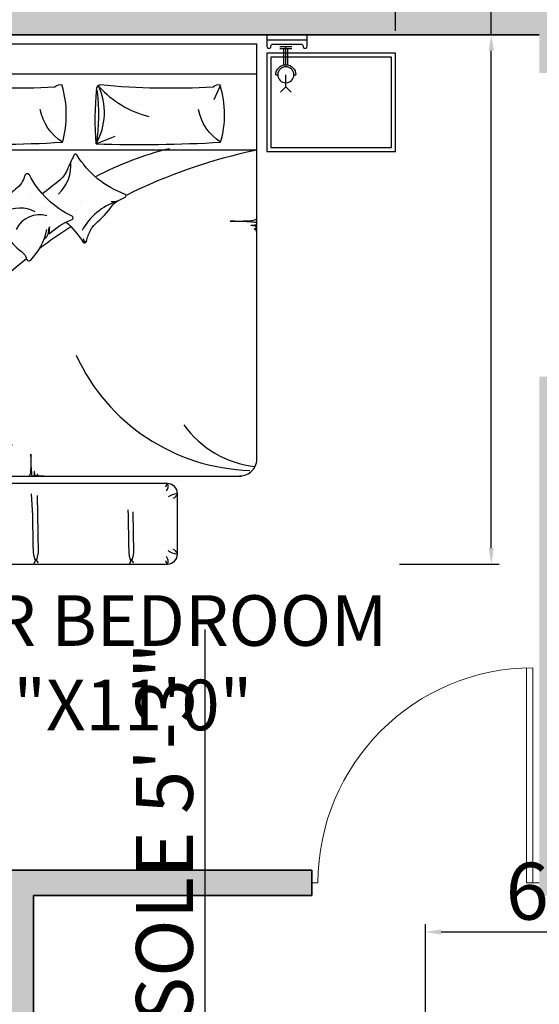
# Model space of a CAD drawing. Units: inches. Extents: x 3592 to 4861, y 1650 to 2243.
# Tile 23 of 30: x 4109 to 4191, y 2003 to 2159. Entities that reach past the tile are written whole.
import ezdxf

# ---------------------------------------------------------------- set-up
doc = ezdxf.new("R2010")
doc.units = ezdxf.units.IN
for name, color, linetype, lineweight in [('A-ANNO-DIMS', 2, 'Continuous', 13), ('A-AREA-IDEN', 7, 'Continuous', 18), ('A-DOOR', 3, 'Continuous', 20), ('A-FURN', 9, 'Continuous', 13), ('A-WALL', 7, 'Continuous', 35)]:
    doc.layers.add(name, color=color, linetype=linetype, lineweight=lineweight)
doc.layers.add('A-WALL-PATT', color=252, linetype='Continuous', lineweight=13, true_color=0x939598)
for name, color, linetype in [('CEIL', 4, 'Continuous'), ('ELEC', 4, 'Continuous'), ('FUR', 42, 'Continuous'), ('wood', 26, 'Continuous')]:
    doc.layers.add(name, color=color, linetype=linetype)
doc.styles.get("Standard").update_dxf_attribs({"font": 'arial.ttf'})
doc.dimstyles.new('ISO-25', dxfattribs={"dimtxt": 9, "dimasz": 2.5, "dimexe": 1.25, "dimexo": 0.625, "dimtad": 1, "dimlunit": 3, "dimtxsty": 'Standard', "dimcen": 2.5, "dimadec": 0, "dimazin": 0, "dimtfac": 1, "dimtmove": 0, "dimatfit": 3, "dimfxl": 1, "dimarcsym": 0})

# ---------------------------------------------------------------- blocks, each defined once
blk = doc.blocks.new('1')
for p, q in [((3628.27, 1890.86), (3628.27, 1924.86)), ((3629.27, 1890.86), (3629.27, 1924.86)), ((3627.27, 1890.86), (3629.27, 1890.86)), ((3662.27, 1890.86), (3663.27, 1890.86))]:
    blk.add_line(p, q)
blk.add_arc((3628.27, 1890.86), 34, 0, 90)
blk = doc.blocks.new('*X20')
at = {"color": 0}
for p, q in [((3155.9, 8182.9), (3155.9, 8182.9)), ((3147.8, 8143.4), (3147.8, 8143.4)), ((3283, 8049.6), (3283, 8049.6)), ((3209.5, 8023.9), (3209.5, 8023.9)), ((3251.6, 7997), (3251.6, 7997)), ((3154.1, 7950.7), (3154.1, 7950.7))]:
    blk.add_line(p, q, dxfattribs=at)
blk = doc.blocks.new('*X19')
at = {"color": 0}
for p, q in [((3155.9, 8182.9), (3155.9, 8182.9)), ((3139.8, 7939.7), (3139.8, 7939.7))]:
    blk.add_line(p, q, dxfattribs=at)
blk = doc.blocks.new('*X18')
at = {"color": 0}
for p, q in [((3155.9, 8182.9), (3155.9, 8182.9)), ((3139.8, 7939.7), (3139.8, 7939.7))]:
    blk.add_line(p, q, dxfattribs=at)
blk = doc.blocks.new('*X17')
at = {"color": 0}
for p, q in [((3163, 7776.2), (3163, 7776.2)), ((3422.2, 7761.3), (3422.2, 7761.3)), ((3244.3, 7698.6), (3244.3, 7698.6)), ((3340.3, 7689.4), (3340.3, 7689.4)), ((3236.2, 7675.7), (3236.2, 7675.7))]:
    blk.add_line(p, q, dxfattribs=at)
blk = doc.blocks.new('BED1')
for p, q in [((0, -1000), (0, 800)), ((150, 800), (0, 800)), ((150, 800), (150, -1000)), ((2058.7, 800), (150, 800)), ((528, 800), (528, -1000)), ((211.8, 614.9), (277.5, 585.4)), ((2537.2, 404.9), (2237.2, 404.9)), ((2187.2, 354.9), (2187.2, -545.1)), ((2587.2, -545.1), (2587.2, 354.9)), ((2566.3, 178.5), (2565.2, 177.4)), ((2582, 188.1), (2565.4, 174.8)), ((2565.4, 174.8), (2585.7, 165.4)), ((2582, -287.1), (2565.4, -300.5)), ((2566.3, -296.8), (2565.2, -297.9)), ((2565.4, -300.5), (2585.7, -309.9)), ((2237.2, -595.1), (2537.2, -595.1)), ((150, -1000), (0, -1000)), ((150, -1000), (2063.5, -1000))]:
    blk.add_line(p, q)
for points in [[(934, 797.9), (930.9, 797.7), (928.3, 797.4), (926.3, 796.9), (924.9, 796.3), (923.8, 795.6), (923.1, 794.8), (922.7, 793.8), (922.5, 792.7), (922.4, 791.5), (922.5, 790.3), (922.6, 789.2), (922.6, 788.3), (922.6, 787.6), (922.4, 787.3), (922, 787.4), (921.4, 787.9), (920.6, 788.9), (919.5, 790.2), (918.4, 791.6), (917.1, 793.1), (915.9, 794.6), (914.6, 796), (913.3, 797.1), (912.2, 797.9), (911.1, 798.3), (910.1, 798.4), (909.2, 798), (908.3, 797.1), (907.5, 795.8), (906.8, 793.9), (906, 791.4), (905.4, 788.5), (904.8, 785.2), (904.2, 781.7), (903.7, 778.4), (903.2, 775.4), (902.8, 772.9), (902.5, 771.3), (902.3, 770.6), (902.1, 771.2), (902, 772.8), (901.8, 775.2), (901.7, 778.1), (901.5, 781.5), (901.2, 785), (900.8, 788.4), (900.2, 791.5), (899.5, 794.1), (898.6, 796.2), (897.6, 797.9), (896.5, 799.2), (895.3, 800), (894.1, 800.5), (893, 800.7), (891.9, 800.5), (890.9, 800.1), (890, 799), (889.1, 797.1), (888.3, 794), (887.6, 789.3), (886.9, 782.9), (886.2, 774.2), (885.5, 763.1), (884.8, 749.5), (884.2, 734.2), (883.6, 718.3), (883, 702.8), (882.5, 688.8), (882, 677.5), (881.7, 669.8), (881.5, 666.9), (881.3, 669.4), (881.3, 676.7), (881.3, 687.8), (881.2, 701.5), (881.1, 716.8), (880.8, 732.6), (880.2, 748), (879.4, 761.8), (878.3, 773.2), (876.9, 782.2), (875.1, 789.2), (872.9, 794.4), (870.3, 798), (869, 799)], [(2150, -913.5), (2150, 723.2)], [(2327.6, 182.3), (2530, 185.9), (2550.8, 181.9), (2561.7, 179), (2566, 176.7), (2566.9, 174.4), (2566.3, 171.9), (2562, 169.2), (2550.3, 166.5), (2527.7, 163.9), (2490.6, 161.8), (2345.5, 160.2), (2317.8, 158.5)], [(494.7, 3.1), (458.9, 95.3)], [(2149.7, -259.9), (2150, -268.4), (2150.1, -274.1), (2150.1, -278.1), (2150, -281.4), (2149.8, -284), (2149.5, -286.1), (2149.1, -287.8), (2148.7, -289), (2148.1, -289.9), (2147.4, -290.5), (2146.6, -290.8), (2145.6, -291), (2144.6, -291), (2143.6, -291), (2142.7, -290.9), (2141.9, -290.9), (2141.4, -290.9), (2141.1, -291), (2141.2, -291.4), (2141.7, -291.9), (2142.5, -292.6), (2143.5, -293.4), (2144.7, -294.4), (2146, -295.4), (2147.2, -296.5), (2148.4, -297.6), (2149.3, -298.6), (2150, -299.6), (2150.3, -300.5), (2150.4, -301.3), (2150, -302.1), (2149.3, -302.8), (2148.2, -303.5), (2146.6, -304.1), (2144.6, -304.7), (2142.1, -305.2), (2139.3, -305.7), (2136.5, -306.2), (2133.7, -306.6), (2131.2, -307), (2129.2, -307.3), (2127.8, -307.6), (2127.3, -307.8), (2127.7, -308), (2129, -308.1), (2131, -308.2), (2133.5, -308.3), (2136.3, -308.5), (2139.2, -308.7), (2142, -309), (2144.6, -309.5), (2146.8, -310.1), (2148.6, -310.9), (2150, -311.7), (2151, -312.7), (2151.7, -313.6), (2152.1, -314.6), (2152.3, -315.6), (2152.2, -316.5), (2151.8, -317.3), (2150.9, -318.1), (2149.3, -318.8), (2146.7, -319.4), (2142.8, -320), (2137.4, -320.6), (2130.2, -321.2), (2121, -321.8), (2109.7, -322.3), (2096.9, -322.9), (2083.6, -323.4), (2070.7, -323.9), (2059.1, -324.3), (2049.6, -324.7), (2043.2, -325), (2040.8, -325.2), (2042.9, -325.3), (2049, -325.3), (2058.2, -325.3), (2069.6, -325.4), (2082.3, -325.5), (2095.6, -325.8), (2108.4, -326.2), (2119.9, -326.8), (2129.4, -327.8), (2136.9, -329), (2142.7, -330.5), (2147, -332.3), (2150, -334.4), (2150.9, -335.6)], [(2246.5, -294.4), (2530, -289.4), (2550.8, -293.4), (2561.7, -296.3), (2566, -298.6), (2566.9, -300.8), (2566.3, -303.4), (2562, -306.1), (2550.3, -308.8), (2527.7, -311.3), (2490.6, -313.5), (2345.5, -315), (2238.6, -321.8)], [(1733.7, -998.3), (1731.1, -998.1), (1729, -997.8), (1727.4, -997.4), (1726.1, -997), (1725.2, -996.4), (1724.7, -995.7), (1724.3, -994.8), (1724.1, -993.9), (1724.1, -992.9), (1724.1, -991.9), (1724.2, -991), (1724.2, -990.2), (1724.2, -989.7), (1724.1, -989.4), (1723.8, -989.5), (1723.2, -990), (1722.5, -990.8), (1721.7, -991.8), (1720.7, -993), (1719.7, -994.3), (1718.6, -995.5), (1717.5, -996.6), (1716.5, -997.6), (1715.5, -998.3), (1714.6, -998.6), (1713.8, -998.6), (1713, -998.3), (1712.3, -997.6), (1711.7, -996.5), (1711, -994.9), (1710.4, -992.9), (1709.9, -990.4), (1709.4, -987.6), (1708.9, -984.8), (1708.5, -982), (1708.1, -979.5), (1707.8, -977.4), (1707.5, -976.1), (1707.3, -975.5), (1707.1, -976), (1707, -977.3), (1706.9, -979.3), (1706.8, -981.8), (1706.7, -984.6), (1706.4, -987.5), (1706.1, -990.3), (1705.6, -992.9), (1705, -995.1), (1704.2, -996.9), (1703.4, -998.3), (1702.4, -999.3), (1701.5, -1000), (1700.5, -1000.4), (1699.6, -1000.6), (1698.7, -1000.4), (1697.8, -1000.1), (1697, -999.2), (1696.3, -997.6), (1695.7, -995), (1695.1, -991.1), (1694.5, -985.7), (1693.9, -978.5), (1693.3, -969.3), (1692.8, -957.9), (1692.2, -945.2), (1691.7, -931.9), (1691.2, -919), (1690.8, -907.4), (1690.4, -897.9), (1690.1, -891.5), (1689.9, -889.1), (1689.8, -891.2), (1689.8, -897.3), (1689.8, -906.5), (1689.7, -917.9), (1689.6, -930.6), (1689.4, -943.8), (1688.9, -956.6), (1688.3, -968.1), (1687.3, -977.6), (1686.1, -985.2), (1684.6, -991), (1682.8, -995.3), (1680.7, -998.3), (1679.6, -999.2)]]:
    blk.add_lwpolyline(points)
for points in [[(489.2, 619.6, 0.144019), (207.6, 617.9, 0.248643)], [(205.5, 619.6, 0.267769), (215.1, 582.4, -0.037739), (204.3, 21.8, 0.684696), (236.7, 5.5, -0.060702), (497.2, 0.1, -0.046649), (225.9, 3.1, -1.318436)], [(497.2, 0.1, 0.021276), (489.2, 619.6, -0.206383), (326.6, 509.4, 0.237198)], [(211.8, 12.8, 0.143972), (361.6, 262.9, 1.292232)], [(886.4, -150, -0.069098), (985, -66.5, 0.658965), (982.1, -48.7, -0.049789), (927.4, -29, -0.103757), (896.6, -5.4, 0.055725), (800.9, 83.3, -0.11866), (782.7, 104.9, 0.016811), (761.6, 143.9, 0.70791), (748.3, 144, -0.16964), (551.9, -96.6, 0.664036), (554, -110.7, 0.023706), (627, -144.7, -0.134834), (683.2, -188, 0.012748), (746.3, -267.4)], [(969.1, -259.1, 0.263265), (936.3, -236.9, -0.026108), (909.2, -233.2, 0.027613), (945.1, -234.2, -0.089259), (872.7, -120, 0.662242), (857.6, -119.3, -0.162037), (651.8, -332.7, 0.676499), (654, -354.5, -0.160513), (722.9, -401.5, 0.07473), (773.5, -450.3, -0.187721), (845.5, -559.9, 0.70791), (858.8, -561.4, -0.010003), (898.6, -497.3, -0.113819), (947.3, -450.2, 0.099539), (1032.5, -372.4, -0.173425), (1070.9, -346.4, 0.589988), (1076.2, -326.1, 0.137312), (923.9, -245.9, 0.137312)], [(205.5, -168.2, 0.267769), (215.1, -205.4, -0.037739), (204.3, -766, 0.684696), (236.7, -782.3, -0.060702), (497.2, -787.7, -0.046649), (225.9, -784.7, -1.318436)], [(489.2, -168.2, 0.144019), (207.6, -169.9, 0.248643)], [(497.2, -787.7, 0.021276), (489.2, -168.2, -0.206383), (326.6, -278.4, 0.237198)], [(1446, -733.4, -0.095039), (652.8, -1001.7)]]:
    blk.add_lwpolyline(points, format="xyb")
for centre, radius, start, end in [((3208.8, 1363.3), 2739.4, 191.8679, 206.3247), ((1608.1, 842.5), 496.3, 305.1901, 354.0206), ((2062.7, 713.7), 86.5, 0, 93.5376), ((1138.6, 793.9), 983.2, 294.6078, 358.3033), ((2237.2, 354.9), 50, 90, 180), ((2321.1, 409.7), 84.5, 185.6196, 217.1396), ((2227.5, 373.5), 32.8, 17.833, 72.8005), ((2546.9, 373.5), 32.8, 107.1995, 162.167), ((2453.3, 409.7), 84.5, 322.8604, 354.3804), ((2537.2, 354.9), 50, 0, 90), ((2098.7, 754.7), 1625, 193.905, 207.8169), ((2201.9, 323.3), 34.8, 50.8413, 114.9586), ((2212.2, 381.5), 36.5, 226.8095, 258.3841), ((2572.5, 323.3), 34.8, 65.0414, 129.1587), ((2562.2, 381.5), 36.5, 281.6159, 313.1905), ((751.8, 88.7), 34.9, 336.8352, 27.7218), ((684.2, 86), 100.3, 353.675, 10.882), ((1074.1, 198.8), 306.1, 197.8602, 241.5122), ((341.4, -277.7), 318.5, 60.7125, 115.009), ((983.7, -79.5), 20.8, 73.7967, 130.4566), ((978.5, -68.6), 14.3, 39.7097, 85.9506), ((602.5, -324), 198.6, 43.2035, 95.0556), ((3208.8, 1363.3), 2739.4, 212.9314, 216.951), ((981.1, -281.8), 131.1, 164.0372, 243.4536), ((980, -379), 163.4, 152.6104, 209.361), ((3208.8, 1363.3), 2739.4, 218.6329, 229.9449), ((2098.7, 754.7), 1625, 226.5887, 246.3156), ((3402.5, -342.9), 1408.5, 182.9917, 205.6819), ((-34.4, -471.2), 376.5, 312.0118, 350.9635), ((2178, -513.5), 33, 286.1827, 338.1386), ((2188.1, -476.2), 73, 269.4513, 322.8027), ((2562.2, -571.8), 36.5, 46.8095, 78.3841), ((2237.2, -545.1), 50, 180, 270), ((2271.1, -580.9), 35.8, 148.9055, 197.5541), ((2546.9, -563.8), 32.8, 197.833, 252.8005), ((2453.3, -600), 84.5, 5.6196, 37.1396), ((2537.2, -545.1), 50, 270, 0), ((2572.5, -513.6), 34.8, 230.8413, 294.9586), ((375.7, -807.4), 128.2, 17.4073, 88.5129), ((341.4, -1065.5), 318.5, 60.7125, 115.009), ((1929.1, -1126), 250.5, 37.8553, 88.4405), ((2063.5, -913.5), 86.5, 270, 0)]:
    blk.add_arc(centre, radius, start, end)
for name in ['*X19', '*X18', '*X20', '*X17']:
    blk.add_blockref(name, (-2425.3, -8101.4))
blk = doc.blocks.new('APLIQ')
at = {"layer": 'ELEC'}
for p, q in [((0, 0.2), (-0.0261, 0.2261)), ((0, 0.2), (0.0261, 0.2261)), ((0, 0.2), (0, 0.14)), ((-0.05, 0.14), (-0.04, 0.14)), ((0.04, 0.14), (0.05, 0.14)), ((-0.01, 0.09), (-0.01, 0.01)), ((0, 0.09), (0, 0)), ((0.01, 0.09), (0.01, 0.01)), ((-0.03, 0.01), (0.03, 0.01)), ((-0.03, 0), (0.03, 0))]:
    blk.add_line(p, q, dxfattribs=at)
blk.add_circle((0, 0.14), 0.04, dxfattribs=at)
blk.add_arc((0, 0.14), 0.05, 180, 0, dxfattribs=at)
blk = doc.blocks.new('A$C68AE1801')
at = {"layer": 'FUR'}
for points in [[(2.5416, 3.18), (2.5416, 2.54), (2.0516, 2.54), (2.0516, 3.18)], [(2.5216, 3.16), (2.5216, 2.56), (2.0716, 2.56), (2.0716, 3.16)], [(2.5416, 0), (2.5416, 0.64), (2.0516, 0.64), (2.0516, 0)], [(2.5216, 0.02), (2.5216, 0.62), (2.0716, 0.62), (2.0716, 0.02)]]:
    blk.add_lwpolyline(points, close=True, dxfattribs=at)
at = {"layer": 'wood'}
for p, q in [((2.6057, 2.74), (2.6057, 2.54)), ((2.6057, 0.44), (2.6057, 0.64))]:
    blk.add_line(p, q, dxfattribs=at)
for points in [[(2.5657, 2.728), (2.5657, 2.732, -0.414214), (2.5737, 2.74), (2.6321, 2.74), (2.6321, 2.54), (2.5737, 2.54, -0.414214), (2.5657, 2.548), (2.5657, 2.552, -0.414214), (2.5737, 2.56), (2.5777, 2.56, 0.414214), (2.5857, 2.568), (2.5857, 2.712, 0.414214), (2.5777, 2.72), (2.5737, 2.72, -0.414214)], [(2.5657, 0.452), (2.5657, 0.448, 0.414214), (2.5737, 0.44), (2.6321, 0.44), (2.6321, 0.64), (2.5737, 0.64, 0.414214), (2.5657, 0.632), (2.5657, 0.628, 0.414214), (2.5737, 0.62), (2.5777, 0.62, -0.414214), (2.5857, 0.612), (2.5857, 0.468, -0.414214), (2.5777, 0.46), (2.5737, 0.46, 0.414214)]]:
    blk.add_lwpolyline(points, format="xyb", close=True, dxfattribs=at)
at = {"layer": 'CEIL', "rotation": 90}
blk.add_blockref('APLIQ', (2.5736, 2.634), dxfattribs=at)
at = {"layer": 'CEIL', "xscale": -1, "rotation": 90}
blk.add_blockref('APLIQ', (2.5736, 0.546), dxfattribs=at)
at = {"layer": 'FUR', "xscale": 0.001, "yscale": 0.001, "zscale": 0.001, "rotation": 180}
blk.add_blockref('BED1', (2.5872, 1.49), dxfattribs=at)
blk = doc.blocks.new('*D150')
at = {"layer": 'A-ANNO-DIMS', "color": 0, "lineweight": -2, "transparency": 16777216}
for p, q in [((4101.85, 2020.28), (4101.85, 2140.68)), ((4100.04, 2020.28), (4103.1, 2020.28)), ((4101.85, 2006.52), (4101.85, 2017.78)), ((4100.04, 2004.02), (4103.1, 2004.02))]:
    blk.add_line(p, q, dxfattribs=at)
at = {"layer": 'A-ANNO-DIMS', "color": 0, "transparency": 16777216}
for points in [[(4101.43, 2017.78), (4102.27, 2017.78), (4101.85, 2020.28)], [(4101.43, 2006.52), (4102.27, 2006.52), (4101.85, 2004.02)]]:
    blk.add_solid(points, dxfattribs=at)
at = {"layer": 'Defpoints', "color": 0, "transparency": 16777216}
for p in [(4099.41, 2020.28), (4101.85, 2020.28), (4099.41, 2004.02)]:
    blk.add_point(p, dxfattribs=at)
at = {"layer": 'A-ANNO-DIMS', "color": 0, "transparency": 16777216, "insert": (4096.57, 2081.73), "char_height": 9, "attachment_point": 5, "rotation": 90}
blk.add_mtext('BASIN 1\'-4 1/2" TYP.', dxfattribs=at)
blk = doc.blocks.new('*D154')
at = {"layer": 'A-ANNO-DIMS', "color": 0, "lineweight": -2, "transparency": 16777216}
for p, q in [((4067.61, 2156.84), (4067.61, 2172.62)), ((4168.62, 2156.84), (4168.62, 2172.62)), ((4067.61, 2171.37), (3930.45, 2171.37)), ((4166.12, 2171.37), (4070.11, 2171.37))]:
    blk.add_line(p, q, dxfattribs=at)
at = {"layer": 'A-ANNO-DIMS', "color": 0, "transparency": 16777216}
for points in [[(4070.11, 2171.79), (4070.11, 2170.95), (4067.61, 2171.37)], [(4166.12, 2171.79), (4166.12, 2170.95), (4168.62, 2171.37)]]:
    blk.add_solid(points, dxfattribs=at)
at = {"layer": 'Defpoints', "color": 0, "transparency": 16777216}
for p in [(4067.61, 2171.37), (4067.61, 2156.22), (4168.62, 2156.22)]:
    blk.add_point(p, dxfattribs=at)
at = {"layer": 'A-ANNO-DIMS', "color": 0, "transparency": 16777216, "insert": (3997.78, 2176.65), "char_height": 9, "attachment_point": 5}
blk.add_mtext('BED GROUP 8\'-5" TYP.', dxfattribs=at)
blk = doc.blocks.new('*D155')
at = {"layer": 'A-ANNO-DIMS', "color": 0, "lineweight": -2, "transparency": 16777216}
for p, q in [((4183.77, 2156.22), (4183.77, 2242.84)), ((4169.25, 2156.22), (4185.02, 2156.22)), ((4183.77, 2075.11), (4183.77, 2153.72)), ((4169.25, 2072.61), (4185.02, 2072.61))]:
    blk.add_line(p, q, dxfattribs=at)
at = {"layer": 'A-ANNO-DIMS', "color": 0, "transparency": 16777216}
for points in [[(4183.36, 2153.72), (4184.19, 2153.72), (4183.77, 2156.22)], [(4183.36, 2075.11), (4184.19, 2075.11), (4183.77, 2072.61)]]:
    blk.add_solid(points, dxfattribs=at)
at = {"layer": 'Defpoints', "color": 0, "transparency": 16777216}
for p in [(4168.62, 2156.22), (4183.77, 2156.22), (4168.62, 2072.61)]:
    blk.add_point(p, dxfattribs=at)
at = {"layer": 'A-ANNO-DIMS', "color": 0, "transparency": 16777216, "insert": (4178.5, 2200.78), "char_height": 9, "attachment_point": 5, "rotation": 90}
blk.add_mtext('6\'-11 1/2" TYP.', dxfattribs=at)
blk = doc.blocks.new('*D165')
at = {"layer": 'A-ANNO-DIMS', "color": 0, "lineweight": -2, "transparency": 16777216}
for p, q in [((4173.35, 1996.55), (4173.35, 2015.72)), ((4247.08, 1996.55), (4247.08, 2015.72)), ((4175.85, 2014.47), (4244.58, 2014.47))]:
    blk.add_line(p, q, dxfattribs=at)
at = {"layer": 'A-ANNO-DIMS', "color": 0, "transparency": 16777216}
for points in [[(4175.85, 2014.88), (4175.85, 2014.05), (4173.35, 2014.47)], [(4244.58, 2014.88), (4244.58, 2014.05), (4247.08, 2014.47)]]:
    blk.add_solid(points, dxfattribs=at)
at = {"layer": 'Defpoints', "color": 0, "transparency": 16777216}
for p in [(4247.08, 2014.47), (4173.35, 1995.93), (4247.08, 1995.93)]:
    blk.add_point(p, dxfattribs=at)
at = {"layer": 'A-ANNO-DIMS', "color": 0, "transparency": 16777216, "insert": (4210.21, 2019.75), "char_height": 9, "attachment_point": 5}
blk.add_mtext('6\'-1 1/2"', dxfattribs=at)
blk = doc.blocks.new('*D168')
at = {"layer": 'A-ANNO-DIMS', "color": 0, "lineweight": -2, "transparency": 16777216}
for p, q in [((4138.54, 1969.72), (4138.54, 2062.26)), ((4129.71, 1969.72), (4139.79, 1969.72)), ((4138.54, 1909.22), (4138.54, 1967.22)), ((4129.71, 1906.72), (4139.79, 1906.72))]:
    blk.add_line(p, q, dxfattribs=at)
at = {"layer": 'A-ANNO-DIMS', "color": 0, "transparency": 16777216}
for points in [[(4138.12, 1967.22), (4138.95, 1967.22), (4138.54, 1969.72)], [(4138.12, 1909.22), (4138.95, 1909.22), (4138.54, 1906.72)]]:
    blk.add_solid(points, dxfattribs=at)
at = {"layer": 'Defpoints', "color": 0, "transparency": 16777216}
for p in [(4129.09, 1969.72), (4138.54, 1969.72), (4129.09, 1906.72)]:
    blk.add_point(p, dxfattribs=at)
at = {"layer": 'A-ANNO-DIMS', "color": 0, "transparency": 16777216, "insert": (4133.25, 2017.24), "char_height": 9, "attachment_point": 5, "rotation": 90}
blk.add_mtext('CONSOLE 5\'-3"', dxfattribs=at)
blk = doc.blocks.new('*D179')
at = {"layer": 'A-ANNO-DIMS', "color": 0, "lineweight": -2, "transparency": 16777216}
for p, q in [((4092.37, 2010.81), (4092.37, 2193.52)), ((4094.87, 2192.27), (4104.87, 2192.27)), ((4107.37, 2020.84), (4107.37, 2193.52)), ((4107.37, 2192.27), (4134.2, 2192.27))]:
    blk.add_line(p, q, dxfattribs=at)
at = {"layer": 'A-ANNO-DIMS', "color": 0, "transparency": 16777216}
for points in [[(4094.87, 2192.69), (4094.87, 2191.85), (4092.37, 2192.27)], [(4104.87, 2192.69), (4104.87, 2191.85), (4107.37, 2192.27)]]:
    blk.add_solid(points, dxfattribs=at)
at = {"layer": 'Defpoints', "color": 0, "transparency": 16777216}
for p in [(4107.37, 2192.27), (4107.37, 2020.22), (4092.37, 2010.18)]:
    blk.add_point(p, dxfattribs=at)
at = {"layer": 'A-ANNO-DIMS', "color": 0, "transparency": 16777216, "insert": (4122.03, 2197.49), "char_height": 9, "attachment_point": 5}
blk.add_mtext('1\'-3"', dxfattribs=at)

msp = doc.modelspace()

# ---------------------------------------------------------------- hatches: boundary and pattern name
at = {"layer": 'A-WALL-PATT'}
h = msp.add_hatch(color=256, dxfattribs=at)
h.dxf.hatch_style = 1
h.paths.add_polyline_path([(4398.37, 2165.219), (4038.37, 2165.219), (4038.37, 1993.219), (4047.37, 1993.219), (4047.37, 2156.219), (4191.37, 2156.219), (4191.37, 2150.219), (4195.37, 2150.219), (4195.37, 2156.219), (4256.37, 2156.219), (4256.37, 2150.219), (4265.37, 2150.219), (4265.37, 2156.219), (4389.37, 2156.219), (4389.37, 2114.219), (4398.37, 2114.219)])
h.paths.add_polyline_path([(4265.37, 2102.219), (4256.37, 2102.219), (4256.37, 2096.219), (4195.37, 2096.219), (4195.37, 2102.219), (4191.37, 2102.219), (4191.37, 2020.219), (4195.37, 2020.219), (4195.37, 2087.219), (4256.37, 2087.219), (4256.37, 2020.219), (4306.37, 2020.219), (4306.37, 2024.219), (4265.37, 2024.219)], flags=17)
h.paths.add_polyline_path([(4398.37, 2066.219), (4389.37, 2066.219), (4389.37, 2024.219), (4348.37, 2024.219), (4348.37, 2020.219), (4389.37, 2020.219), (4389.37, 1989.719), (4398.37, 1989.719)])
h.paths.add_polyline_path([(4398.37, 1941.719), (4389.37, 1941.719), (4389.37, 1911.219), (4301.37, 1911.219), (4301.37, 1907.219), (4389.37, 1907.219), (4389.37, 1865.219), (4398.37, 1865.219)])
h.paths.add_polyline_path([(4398.37, 1817.219), (4389.37, 1817.219), (4389.37, 1775.219), (4265.37, 1775.219), (4265.37, 1911.219), (4256.37, 1911.219), (4256.37, 1817.219), (4220.87, 1817.219), (4220.87, 1808.219), (4256.37, 1808.219), (4256.37, 1766.219), (4389.37, 1766.219), (4389.37, 1694.219), (4256.37, 1694.219), (4256.37, 1685.219), (4398.37, 1685.219)])
h.paths.add_polyline_path([(4178.87, 1817.219), (4077.37, 1817.219), (4077.37, 1808.219), (4178.87, 1808.219)])
h.paths.add_polyline_path([(4111.37, 2020.219), (4155.37, 2020.219), (4155.37, 2024.219), (4077.37, 2024.219), (4077.37, 2020.219), (4107.37, 2020.219), (4107.37, 1942.219), (4047.37, 1942.219), (4047.37, 1969.219), (4038.37, 1969.219), (4038.37, 1911.219), (4047.37, 1911.219), (4047.37, 1938.219), (4107.37, 1938.219), (4107.37, 1860.219), (4077.37, 1860.219), (4077.37, 1856.219), (4111.37, 1856.219)])
h.paths.add_polyline_path([(4047.37, 1887.219), (4038.37, 1887.219), (4038.37, 1685.219), (4152.37, 1685.219), (4152.37, 1715.219), (4143.37, 1715.219), (4143.37, 1694.219), (4047.37, 1694.219)])
h.paths.add_polyline_path([(4152.37, 1772.219), (4143.37, 1772.219), (4143.37, 1751.219), (4152.37, 1751.219)], flags=17)

# ---------------------------------------------------------------- linework, layer by layer
at = {"layer": 'A-WALL'}
for p, q in [((4047.37, 2156.219), (4191.37, 2156.219)), ((4077.37, 2024.219), (4155.37, 2024.219)), ((4155.37, 2020.219), (4155.37, 2024.219)), ((4111.37, 2020.219), (4155.37, 2020.219)), ((4111.37, 1856.219), (4111.37, 2020.219))]:
    msp.add_line(p, q, dxfattribs=at)

# ---------------------------------------------------------------- block references
at = {"layer": 'A-DOOR', "xscale": -1}
msp.add_blockref('1', (7818.637, 131.354), dxfattribs=at)
at = {"layer": 'A-FURN', "xscale": 31.7658940618111, "yscale": 31.7658940618111, "zscale": 31.7658940618111, "rotation": 90}
msp.add_blockref('A$C68AE1801', (4168.621, 2072.607), dxfattribs=at)

# ---------------------------------------------------------------- texts
at = {"layer": 'A-AREA-IDEN', "insert": (4069.864, 2067.679), "char_height": 8, "attachment_point": 1}
msp.add_mtext_dynamic_manual_height_columns('MASTER BEDROOM\\P       12\'0"X11\'0"', width=121.44943, gutter_width=12.5, heights=[0], dxfattribs=at)

# ---------------------------------------------------------------- dimensions: what is measured, and where the dimension line sits
at = {"layer": 'A-ANNO-DIMS'}
for base, p1, p2, angle, text, picture, middle in [((4183.774, 2156.219), (4168.621, 2072.607), (4168.621, 2156.219), 90, '<> TYP.', '*D155', (4178.495, 2200.78)), ((4067.606, 2171.371), (4168.621, 2156.219), (4067.606, 2156.219), 180, 'BED GROUP <> TYP.', '*D154', (3997.779, 2176.653)), ((4101.85, 2020.278), (4099.412, 2004.022), (4099.412, 2020.278), 90, 'BASIN <> TYP.', '*D150', (4096.571, 2081.731)), ((4138.535, 1969.715), (4129.086, 1906.723), (4129.086, 1969.715), 90, 'CONSOLE <>', '*D168', (4133.25, 2017.238))]:
    dim = msp.add_linear_dim(base=base, p1=p1, p2=p2, angle=angle, text=text, dimstyle='ISO-25', override={"dimdec": 1, "dimlfac": 1, "dimrnd": 0, "dimzin": 1, "dimdsep": 46, "dimlunit": 4, "dimfrac": 2}, dxfattribs=at)
    dim.commit()
    dim.dimension.update_dxf_attribs({"geometry": picture, "text_midpoint": middle})
for base, p1, p2, picture, middle in [((4107.37, 2192.269), (4092.37, 2010.184), (4107.37, 2020.219), '*D179', (4122.033, 2197.492)), ((4247.079, 2014.467), (4173.347, 1995.926), (4247.079, 1995.926), '*D165', (4210.213, 2019.746))]:
    dim = msp.add_linear_dim(base=base, p1=p1, p2=p2, dimstyle='ISO-25', override={"dimdec": 1, "dimlfac": 1, "dimrnd": 0, "dimzin": 1, "dimdsep": 46, "dimlunit": 4, "dimfrac": 2}, dxfattribs=at)
    dim.commit()
    dim.dimension.update_dxf_attribs({"geometry": picture, "text_midpoint": middle})

doc.saveas('drawing.dxf')
